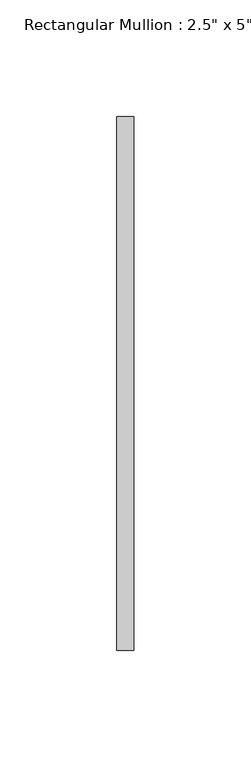
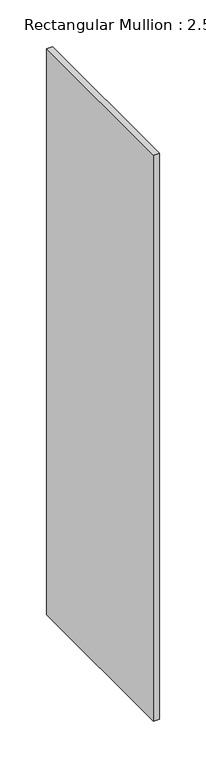
"""IFC4 building model written with IfcOpenShell, lengths in millimetres: member geometry."""

from ifc_helpers import new_model, si_unit, frame, origin, place, context, project, spatial, polyline, outline, extrude, source, transform, mapped, element, save


def member_446da441(model_context):
    return source(origin(), model_context, "Body", "SweptSolid", [
        extrude(outline(polyline([(0.0, 114.3), (0.0, -114.3), (-7.239, -114.3), (-7.239, 114.3), (0.0, 114.3)])), frame((0.0, 0.0, -738.4415), z_axis=(0.0, 0.0, 1.0), x_axis=(1.0, 0.0, 0.0)), (0.0, 0.0, 1.0), 738.4415),
    ])


if __name__ == "__main__":
    model = new_model("IFC4")
    model_context = context("Model", 3, world=origin())
    ifc_project = project(units=[si_unit("LENGTHUNIT", "METRE", prefix="MILLI")], contexts=[model_context])
    site = spatial("IfcSite", under=ifc_project)
    building = spatial("IfcBuilding", under=site)
    placement = place(None, origin())
    member_shape = member_446da441(model_context)
    element("IfcMember", 1, ObjectType="Rectangular Mullion : 2.5\" x 5\" rectangular", at=placement, inside=building, context=model_context, shape_type="MappedRepresentation", body=[
        mapped(member_shape, transform((0.0, 0.0, 0.0), x_axis=(1.0, 0.0, 0.0), y_axis=(0.0, 1.0, 0.0), z_axis=(0.0, 0.0, 1.0))),
    ])
    save(model, "model.ifc")

# Revit data of these elements
# Type "Rectangular Mullion : 2.5\" x 5\" rectangular"
#   built-in parameter 1007304 = 0.75 (stored number, unit not read)
#   built-in parameter 1007301 = 0.011875 (stored number, unit not read)
#   built-in parameter 1007300 = 0.011875 (stored number, unit not read)
# Element 1 (IfcMember, "Rectangular Mullion : 2.5\" x 5\" rectangular")
#   Materials on its faces: "WINDOW GLASS MATERIAL"
# Materials
#   "WINDOW GLASS MATERIAL": class "Generic", colour RGB 120 120 120, transparency 0, Cost = 0
